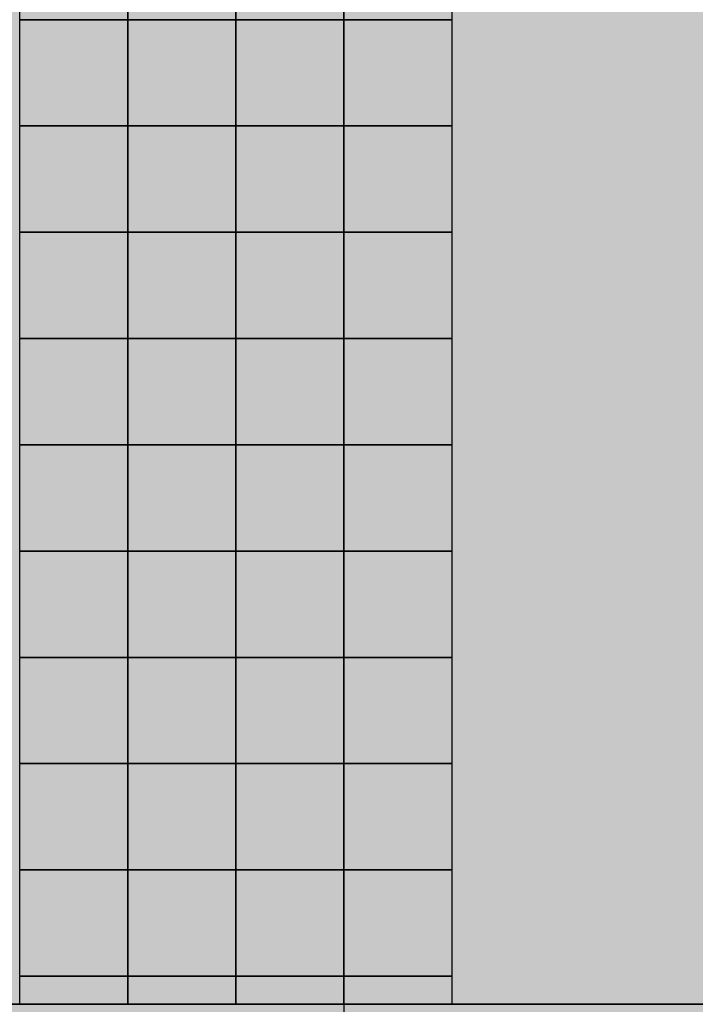
# Model space of a CAD drawing. Units: feet. Extents: x 2695 to 2912, y 795 to 1139.
# Tile 39 of 83: x 2731 to 2769, y 937 to 993. Entities that reach past the tile are written whole.
import ezdxf

# ---------------------------------------------------------------- set-up
doc = ezdxf.new("R2010")
doc.units = ezdxf.units.FT
for name, color, linetype, lineweight in [('A-ELEV', 7, 'Continuous', 35), ('A-ELEV-PATT', 252, 'Continuous', 13), ('A-GLAZ', 4, 'Continuous', 25), ('A-GLAZ-PATT', 254, 'Continuous', 13)]:
    doc.layers.add(name, color=color, linetype=linetype, lineweight=lineweight)

msp = doc.modelspace()

# ---------------------------------------------------------------- hatches: boundary and pattern name
at = {"layer": 'A-ELEV-PATT'}
h = msp.add_hatch(color=256, dxfattribs=at)
h.set_gradient(color1=(255, 255, 255), tint=1)
h.paths.add_polyline_path([(2770.6361, 1122.9306), (2710.6361, 1122.9306), (2710.6361, 1118.4096), (2770.6361, 1118.4096)])
h.paths.add_polyline_path([(2890.6361, 1107.8588), (2770.6361, 1107.8588), (2770.6361, 1103.3378), (2890.6361, 1103.3378)])
h.paths.add_polyline_path([(2890.6361, 1062.9306), (2710.6361, 1062.9306), (2710.6361, 1056.9306), (2710.6361, 936.9306), (2710.6361, 924.3105), (2716.5358, 924.3105), (2890.6361, 924.3105), (2890.6361, 936.9306), (2715.8852, 936.9306), (2715.8852, 1050.3105), (2890.6361, 1050.3105)])
h.paths.add_polyline_path([(2716.5358, 924.3105), (2710.6361, 924.3105), (2710.6361, 810.9306), (2716.5358, 810.9306)])
h = msp.add_hatch(color=256, dxfattribs=at)
h.set_gradient(color1=(147, 149, 152), color2=(147, 149, 152), tint=1)
h.paths.add_polyline_path([(2770.6361, 1118.4096), (2710.6361, 1118.4096), (2710.6361, 1062.9306), (2770.6361, 1062.9306)])
h.paths.add_polyline_path([(2890.6361, 1103.3378), (2770.6361, 1103.3378), (2770.6361, 1062.9306), (2890.6361, 1062.9306)])
h.paths.add_polyline_path([(2730.7081, 1048.1052), (2755.1125, 1048.1052), (2755.1125, 936.9306), (2770.6361, 936.9306), (2770.6361, 1050.3105), (2715.8852, 1050.3105), (2715.8852, 936.9306), (2730.7081, 936.9306)])
h.paths.add_polyline_path([(2890.6361, 1050.3105), (2770.6361, 1050.3105), (2770.6361, 971.9673), (2778.0341, 971.9673), (2778.0341, 1020.8235), (2843.575, 1020.8235), (2843.575, 971.9673), (2890.6361, 971.9673)])
h.paths.add_polyline_path([(2888.1882, 970.7156), (2843.575, 970.7156), (2843.575, 964.8267), (2888.1882, 964.8267)])
h.paths.add_polyline_path([(2888.1882, 964.1328), (2843.575, 964.1328), (2843.575, 956.614), (2888.1882, 956.614)])
h.paths.add_polyline_path([(2888.1882, 955.9202), (2843.575, 955.9202), (2843.575, 949.2892), (2888.1882, 949.2892)])
h.paths.add_polyline_path([(2888.1882, 948.5954), (2843.575, 948.5954), (2843.575, 941.3507), (2888.1882, 941.3507)])
h.paths.add_polyline_path([(2888.1882, 940.6569), (2843.575, 940.6569), (2843.575, 936.9306), (2888.1882, 936.9306)])
h.paths.add_polyline_path([(2890.6361, 970.7156), (2888.9368, 970.7156), (2888.9368, 964.8267), (2890.6361, 964.8267)])
h.paths.add_polyline_path([(2890.6361, 964.1328), (2888.9368, 964.1328), (2888.9368, 956.614), (2890.6361, 956.614)])
h.paths.add_polyline_path([(2890.6361, 955.9202), (2888.9368, 955.9202), (2888.9368, 949.2892), (2890.6361, 949.2892)])
h.paths.add_polyline_path([(2890.6361, 940.6569), (2888.9368, 940.6569), (2888.9368, 936.9306), (2890.6361, 936.9306)])
h.paths.add_polyline_path([(2890.6361, 948.5954), (2888.9368, 948.5954), (2888.9368, 941.3507), (2890.6361, 941.3507)])
h.paths.add_polyline_path([(2772.5216, 970.7156), (2770.6361, 970.7156), (2770.6361, 964.8267), (2772.5216, 964.8267)])
h.paths.add_polyline_path([(2772.5216, 964.1328), (2770.6361, 964.1328), (2770.6361, 956.614), (2772.5216, 956.614)])
h.paths.add_polyline_path([(2772.5216, 955.9202), (2770.6361, 955.9202), (2770.6361, 949.2892), (2772.5216, 949.2892)])
h.paths.add_polyline_path([(2772.5216, 948.5954), (2770.6361, 948.5954), (2770.6361, 941.3507), (2772.5216, 941.3507)])
h.paths.add_polyline_path([(2772.5216, 940.6569), (2770.6361, 940.6569), (2770.6361, 936.9306), (2772.5216, 936.9306)])
h.paths.add_polyline_path([(2778.0341, 940.6569), (2773.2702, 940.6569), (2773.2702, 936.9306), (2778.0341, 936.9306)])
h.paths.add_polyline_path([(2778.0341, 970.7156), (2773.2702, 970.7156), (2773.2702, 964.8267), (2778.0341, 964.8267)])
h.paths.add_polyline_path([(2778.0341, 964.1328), (2773.2702, 964.1328), (2773.2702, 956.614), (2778.0341, 956.614)])
h.paths.add_polyline_path([(2778.0341, 955.9202), (2773.2702, 955.9202), (2773.2702, 949.2892), (2778.0341, 949.2892)])
h.paths.add_polyline_path([(2778.0341, 948.5954), (2773.2702, 948.5954), (2773.2702, 941.3507), (2778.0341, 941.3507)])
h.paths.add_polyline_path([(2810.0407, 940.6569), (2780.0341, 940.6569), (2780.0341, 936.9306), (2810.0407, 936.9306)])
h.paths.add_polyline_path([(2890.6361, 924.3105), (2770.6361, 924.3105), (2770.6361, 810.9306), (2773.5029, 810.9306), (2773.5029, 905.5143), (2805.9398, 905.5143), (2838.3767, 905.5143), (2838.3767, 810.9306), (2890.6361, 810.9306)])
at = {"layer": 'A-GLAZ-PATT'}
h = msp.add_hatch(color=256, dxfattribs=at)
h.set_gradient(color1=(153, 185, 219), color2=(153, 185, 219))
h.paths.add_polyline_path([(2736.8092, 1048.1052), (2730.7081, 1048.1052), (2730.7081, 1046.5179), (2736.8092, 1046.5179)])
h.paths.add_polyline_path([(2742.9103, 1048.1052), (2736.8092, 1048.1052), (2736.8092, 1046.5179), (2742.9103, 1046.5179)])
h.paths.add_polyline_path([(2749.0114, 1048.1052), (2742.9103, 1048.1052), (2742.9103, 1046.5179), (2749.0114, 1046.5179)])
h.paths.add_polyline_path([(2755.1125, 1048.1052), (2749.0114, 1048.1052), (2749.0114, 1046.5179), (2755.1125, 1046.5179)])
h.paths.add_polyline_path([(2755.1125, 1046.5179), (2749.0114, 1046.5179), (2749.0114, 1040.5179), (2755.1125, 1040.5179)])
h.paths.add_polyline_path([(2749.0114, 1046.5179), (2742.9103, 1046.5179), (2742.9103, 1040.5179), (2749.0114, 1040.5179)])
h.paths.add_polyline_path([(2736.8092, 1046.5179), (2730.7081, 1046.5179), (2730.7081, 1040.5179), (2736.8092, 1040.5179)])
h.paths.add_polyline_path([(2742.9103, 1046.5179), (2736.8092, 1046.5179), (2736.8092, 1040.5179), (2742.9103, 1040.5179)])
h.paths.add_polyline_path([(2736.8092, 1040.5179), (2730.7081, 1040.5179), (2730.7081, 1034.5179), (2736.8092, 1034.5179)])
h.paths.add_polyline_path([(2742.9103, 1040.5179), (2736.8092, 1040.5179), (2736.8092, 1034.5179), (2742.9103, 1034.5179)])
h.paths.add_polyline_path([(2749.0114, 1040.5179), (2742.9103, 1040.5179), (2742.9103, 1034.5179), (2749.0114, 1034.5179)])
h.paths.add_polyline_path([(2755.1125, 1040.5179), (2749.0114, 1040.5179), (2749.0114, 1034.5179), (2755.1125, 1034.5179)])
h.paths.add_polyline_path([(2736.8092, 1034.5179), (2730.7081, 1034.5179), (2730.7081, 1028.5179), (2736.8092, 1028.5179)])
h.paths.add_polyline_path([(2749.0114, 1034.5179), (2742.9103, 1034.5179), (2742.9103, 1028.5179), (2749.0114, 1028.5179)])
h.paths.add_polyline_path([(2742.9103, 1034.5179), (2736.8092, 1034.5179), (2736.8092, 1028.5179), (2742.9103, 1028.5179)])
h.paths.add_polyline_path([(2755.1125, 1034.5179), (2749.0114, 1034.5179), (2749.0114, 1028.5179), (2755.1125, 1028.5179)])
h.paths.add_polyline_path([(2755.1125, 1028.5179), (2749.0114, 1028.5179), (2749.0114, 1022.5179), (2755.1125, 1022.5179)])
h.paths.add_polyline_path([(2749.0114, 1028.5179), (2742.9103, 1028.5179), (2742.9103, 1022.5179), (2749.0114, 1022.5179)])
h.paths.add_polyline_path([(2742.9103, 1028.5179), (2736.8092, 1028.5179), (2736.8092, 1022.5179), (2742.9103, 1022.5179)])
h.paths.add_polyline_path([(2736.8092, 1028.5179), (2730.7081, 1028.5179), (2730.7081, 1022.5179), (2736.8092, 1022.5179)])
h.paths.add_polyline_path([(2736.8092, 1022.5179), (2730.7081, 1022.5179), (2730.7081, 1016.5179), (2736.8092, 1016.5179)])
h.paths.add_polyline_path([(2742.9103, 1022.5179), (2736.8092, 1022.5179), (2736.8092, 1016.5179), (2742.9103, 1016.5179)])
h.paths.add_polyline_path([(2749.0114, 1022.5179), (2742.9103, 1022.5179), (2742.9103, 1016.5179), (2749.0114, 1016.5179)])
h.paths.add_polyline_path([(2755.1125, 1022.5179), (2749.0114, 1022.5179), (2749.0114, 1016.5179), (2755.1125, 1016.5179)])
h.paths.add_polyline_path([(2736.8092, 1016.5179), (2730.7081, 1016.5179), (2730.7081, 1010.5179), (2736.8092, 1010.5179)])
h.paths.add_polyline_path([(2742.9103, 1016.5179), (2736.8092, 1016.5179), (2736.8092, 1010.5179), (2742.9103, 1010.5179)])
h.paths.add_polyline_path([(2749.0114, 1016.5179), (2742.9103, 1016.5179), (2742.9103, 1010.5179), (2749.0114, 1010.5179)])
h.paths.add_polyline_path([(2755.1125, 1016.5179), (2749.0114, 1016.5179), (2749.0114, 1010.5179), (2755.1125, 1010.5179)])
h.paths.add_polyline_path([(2755.1125, 1010.5179), (2749.0114, 1010.5179), (2749.0114, 1004.5179), (2755.1125, 1004.5179)])
h.paths.add_polyline_path([(2749.0114, 1010.5179), (2742.9103, 1010.5179), (2742.9103, 1004.5179), (2749.0114, 1004.5179)])
h.paths.add_polyline_path([(2742.9103, 1010.5179), (2736.8092, 1010.5179), (2736.8092, 1004.5179), (2742.9103, 1004.5179)])
h.paths.add_polyline_path([(2736.8092, 1010.5179), (2730.7081, 1010.5179), (2730.7081, 1004.5179), (2736.8092, 1004.5179)])
h.paths.add_polyline_path([(2736.8092, 1004.5179), (2730.7081, 1004.5179), (2730.7081, 998.5179), (2736.8092, 998.5179)])
h.paths.add_polyline_path([(2742.9103, 1004.5179), (2736.8092, 1004.5179), (2736.8092, 998.5179), (2742.9103, 998.5179)])
h.paths.add_polyline_path([(2749.0114, 1004.5179), (2742.9103, 1004.5179), (2742.9103, 998.5179), (2749.0114, 998.5179)])
h.paths.add_polyline_path([(2755.1125, 1004.5179), (2749.0114, 1004.5179), (2749.0114, 998.5179), (2755.1125, 998.5179)])
h.paths.add_polyline_path([(2755.1125, 998.5179), (2749.0114, 998.5179), (2749.0114, 992.5179), (2755.1125, 992.5179)])
h.paths.add_polyline_path([(2749.0114, 998.5179), (2742.9103, 998.5179), (2742.9103, 992.5179), (2749.0114, 992.5179)])
h.paths.add_polyline_path([(2742.9103, 998.5179), (2736.8092, 998.5179), (2736.8092, 992.5179), (2742.9103, 992.5179)])
h.paths.add_polyline_path([(2736.8092, 998.5179), (2730.7081, 998.5179), (2730.7081, 992.5179), (2736.8092, 992.5179)])
h.paths.add_polyline_path([(2736.8092, 992.5179), (2730.7081, 992.5179), (2730.7081, 986.5179), (2736.8092, 986.5179)])
h.paths.add_polyline_path([(2742.9103, 992.5179), (2736.8092, 992.5179), (2736.8092, 986.5179), (2742.9103, 986.5179)])
h.paths.add_polyline_path([(2749.0114, 992.5179), (2742.9103, 992.5179), (2742.9103, 986.5179), (2749.0114, 986.5179)])
h.paths.add_polyline_path([(2755.1125, 992.5179), (2749.0114, 992.5179), (2749.0114, 986.5179), (2755.1125, 986.5179)])
h.paths.add_polyline_path([(2755.1125, 986.5179), (2749.0114, 986.5179), (2749.0114, 980.5179), (2755.1125, 980.5179)])
h.paths.add_polyline_path([(2749.0114, 986.5179), (2742.9103, 986.5179), (2742.9103, 980.5179), (2749.0114, 980.5179)])
h.paths.add_polyline_path([(2742.9103, 986.5179), (2736.8092, 986.5179), (2736.8092, 980.5179), (2742.9103, 980.5179)])
h.paths.add_polyline_path([(2736.8092, 986.5179), (2730.7081, 986.5179), (2730.7081, 980.5179), (2736.8092, 980.5179)])
h.paths.add_polyline_path([(2755.1125, 980.5179), (2749.0114, 980.5179), (2749.0114, 974.5179), (2755.1125, 974.5179)])
h.paths.add_polyline_path([(2749.0114, 980.5179), (2742.9103, 980.5179), (2742.9103, 974.5179), (2749.0114, 974.5179)])
h.paths.add_polyline_path([(2736.8092, 980.5179), (2730.7081, 980.5179), (2730.7081, 974.5179), (2736.8092, 974.5179)])
h.paths.add_polyline_path([(2742.9103, 980.5179), (2736.8092, 980.5179), (2736.8092, 974.5179), (2742.9103, 974.5179)])
h.paths.add_polyline_path([(2736.8092, 974.5179), (2730.7081, 974.5179), (2730.7081, 968.5179), (2736.8092, 968.5179)])
h.paths.add_polyline_path([(2742.9103, 974.5179), (2736.8092, 974.5179), (2736.8092, 968.5179), (2742.9103, 968.5179)])
h.paths.add_polyline_path([(2755.1125, 974.5179), (2749.0114, 974.5179), (2749.0114, 968.5179), (2755.1125, 968.5179)])
h.paths.add_polyline_path([(2749.0114, 974.5179), (2742.9103, 974.5179), (2742.9103, 968.5179), (2749.0114, 968.5179)])
h.paths.add_polyline_path([(2736.8092, 968.5179), (2730.7081, 968.5179), (2730.7081, 962.5179), (2736.8092, 962.5179)])
h.paths.add_polyline_path([(2742.9103, 968.5179), (2736.8092, 968.5179), (2736.8092, 962.5179), (2742.9103, 962.5179)])
h.paths.add_polyline_path([(2749.0114, 968.5179), (2742.9103, 968.5179), (2742.9103, 962.5179), (2749.0114, 962.5179)])
h.paths.add_polyline_path([(2755.1125, 968.5179), (2749.0114, 968.5179), (2749.0114, 962.5179), (2755.1125, 962.5179)])
h.paths.add_polyline_path([(2755.1125, 962.5179), (2749.0114, 962.5179), (2749.0114, 956.5179), (2755.1125, 956.5179)])
h.paths.add_polyline_path([(2749.0114, 962.5179), (2742.9103, 962.5179), (2742.9103, 956.5179), (2749.0114, 956.5179)])
h.paths.add_polyline_path([(2742.9103, 962.5179), (2736.8092, 962.5179), (2736.8092, 956.5179), (2742.9103, 956.5179)])
h.paths.add_polyline_path([(2736.8092, 962.5179), (2730.7081, 962.5179), (2730.7081, 956.5179), (2736.8092, 956.5179)])
h.paths.add_polyline_path([(2736.8092, 956.5179), (2730.7081, 956.5179), (2730.7081, 950.5179), (2736.8092, 950.5179)])
h.paths.add_polyline_path([(2742.9103, 956.5179), (2736.8092, 956.5179), (2736.8092, 950.5179), (2742.9103, 950.5179)])
h.paths.add_polyline_path([(2749.0114, 956.5179), (2742.9103, 956.5179), (2742.9103, 950.5179), (2749.0114, 950.5179)])
h.paths.add_polyline_path([(2755.1125, 956.5179), (2749.0114, 956.5179), (2749.0114, 950.5179), (2755.1125, 950.5179)])
h.paths.add_polyline_path([(2755.1125, 950.5179), (2749.0114, 950.5179), (2749.0114, 944.5179), (2755.1125, 944.5179)])
h.paths.add_polyline_path([(2749.0114, 950.5179), (2742.9103, 950.5179), (2742.9103, 944.5179), (2749.0114, 944.5179)])
h.paths.add_polyline_path([(2742.9103, 950.5179), (2736.8092, 950.5179), (2736.8092, 944.5179), (2742.9103, 944.5179)])
h.paths.add_polyline_path([(2736.8092, 950.5179), (2730.7081, 950.5179), (2730.7081, 944.5179), (2736.8092, 944.5179)])
h.paths.add_polyline_path([(2736.8092, 944.5179), (2730.7081, 944.5179), (2730.7081, 938.5179), (2736.8092, 938.5179)])
h.paths.add_polyline_path([(2742.9103, 944.5179), (2736.8092, 944.5179), (2736.8092, 938.5179), (2742.9103, 938.5179)])
h.paths.add_polyline_path([(2749.0114, 944.5179), (2742.9103, 944.5179), (2742.9103, 938.5179), (2749.0114, 938.5179)])
h.paths.add_polyline_path([(2755.1125, 944.5179), (2749.0114, 944.5179), (2749.0114, 938.5179), (2755.1125, 938.5179)])
h.paths.add_polyline_path([(2755.1125, 938.5179), (2749.0114, 938.5179), (2749.0114, 936.9306), (2755.1125, 936.9306)])
h.paths.add_polyline_path([(2749.0114, 938.5179), (2742.9103, 938.5179), (2742.9103, 936.9306), (2749.0114, 936.9306)])
h.paths.add_polyline_path([(2742.9103, 938.5179), (2736.8092, 938.5179), (2736.8092, 936.9306), (2742.9103, 936.9306)])
h.paths.add_polyline_path([(2736.8092, 938.5179), (2730.7081, 938.5179), (2730.7081, 936.9306), (2736.8092, 936.9306)])

# ---------------------------------------------------------------- linework, layer by layer
at = {"layer": 'A-ELEV'}
msp.add_line((2715.8852, 936.9306), (2890.6361, 936.9306), dxfattribs=at)
msp.add_line((2715.8852, 936.9306), (2890.6361, 936.9306), dxfattribs=at)
at = {"layer": 'A-GLAZ'}
for p, q in [((2736.8092, 936.9306), (2736.8092, 1048.1052)), ((2742.9103, 936.9306), (2742.9103, 1048.1052)), ((2749.0114, 936.9306), (2749.0114, 1048.1052)), ((2749.0114, 1048.1052), (2749.0114, 935.6966)), ((2730.7081, 992.5179), (2755.1125, 992.5179)), ((2730.7081, 986.5179), (2755.1125, 986.5179)), ((2730.7081, 980.5179), (2755.1125, 980.5179)), ((2730.7081, 974.5179), (2755.1125, 974.5179)), ((2730.7081, 968.5179), (2755.1125, 968.5179)), ((2730.7081, 962.5179), (2755.1125, 962.5179)), ((2730.7081, 956.5179), (2755.1125, 956.5179)), ((2730.7081, 950.5179), (2755.1125, 950.5179)), ((2730.7081, 944.5179), (2755.1125, 944.5179)), ((2730.7081, 938.5179), (2755.1125, 938.5179))]:
    msp.add_line(p, q, dxfattribs=at)
msp.add_lwpolyline([(2730.7081, 936.9306), (2730.7081, 1048.1052), (2755.1125, 1048.1052), (2755.1125, 936.9306)], dxfattribs=at)
for points in [[(2730.7081, 1048.1052), (2755.1125, 1048.1052), (2755.1125, 936.9306), (2730.7081, 936.9306)], [(2736.8092, 1048.1052), (2736.8092, 1048.1052), (2736.8092, 936.9306), (2736.8092, 936.9306)], [(2742.9103, 1048.1052), (2742.9103, 1048.1052), (2742.9103, 936.9306), (2742.9103, 936.9306)], [(2749.0114, 1048.1052), (2749.0114, 1048.1052), (2749.0114, 936.9306), (2749.0114, 936.9306)], [(2730.7081, 992.5179), (2755.1125, 992.5179), (2755.1125, 992.5179), (2730.7081, 992.5179)], [(2730.7081, 986.5179), (2755.1125, 986.5179), (2755.1125, 986.5179), (2730.7081, 986.5179)], [(2730.7081, 980.5179), (2755.1125, 980.5179), (2755.1125, 980.5179), (2730.7081, 980.5179)], [(2730.7081, 974.5179), (2755.1125, 974.5179), (2755.1125, 974.5179), (2730.7081, 974.5179)], [(2730.7081, 968.5179), (2755.1125, 968.5179), (2755.1125, 968.5179), (2730.7081, 968.5179)], [(2730.7081, 962.5179), (2755.1125, 962.5179), (2755.1125, 962.5179), (2730.7081, 962.5179)], [(2730.7081, 956.5179), (2755.1125, 956.5179), (2755.1125, 956.5179), (2730.7081, 956.5179)], [(2730.7081, 950.5179), (2755.1125, 950.5179), (2755.1125, 950.5179), (2730.7081, 950.5179)], [(2730.7081, 944.5179), (2755.1125, 944.5179), (2755.1125, 944.5179), (2730.7081, 944.5179)], [(2730.7081, 938.5179), (2755.1125, 938.5179), (2755.1125, 938.5179), (2730.7081, 938.5179)]]:
    msp.add_lwpolyline(points, close=True, dxfattribs=at)

doc.saveas('drawing.dxf')
